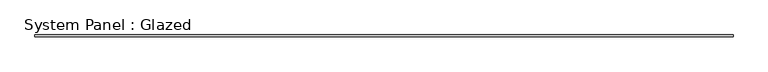
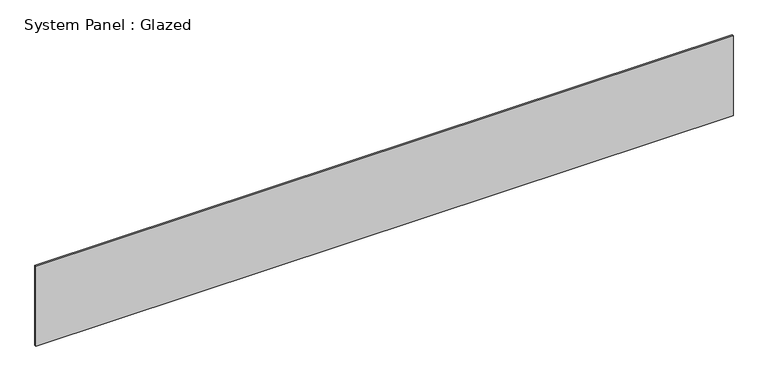
"""IFC4 building model written with IfcOpenShell, lengths in millimetres: plate geometry, System Panel : Glazed."""

from ifc_helpers import new_model, si_unit, origin, origin_with_axes, place, context, project, spatial, polyline, outline, extrude, source, transform, mapped, element, save


def system_panel_glazed_4fccefc8(model_context):
    return source(origin(), model_context, "Body", "SweptSolid", [
        extrude(outline(polyline([(5041.9, 19.05), (-5041.9, 19.05), (-5041.9, 44.45), (5041.9, 44.45), (5041.9, 19.05)])), origin_with_axes(), (0.0, 0.0, 1.0), 1219.2),
    ])


if __name__ == "__main__":
    model = new_model("IFC4")
    model_context = context("Model", 3, world=origin())
    ifc_project = project(units=[si_unit("LENGTHUNIT", "METRE", prefix="MILLI")], contexts=[model_context])
    site = spatial("IfcSite", under=ifc_project)
    building = spatial("IfcBuilding", under=site)
    placement = place(None, origin())
    system_panel_glazed_shape = system_panel_glazed_4fccefc8(model_context)
    element("IfcPlate", 1, ObjectType="System Panel : Glazed", at=placement, inside=building, context=model_context, shape_type="MappedRepresentation", body=[
        mapped(system_panel_glazed_shape, transform((0.0, 0.0, 0.0), x_axis=(1.0, 0.0, 0.0), y_axis=(0.0, 1.0, 0.0), z_axis=(0.0, 0.0, 1.0))),
    ])
    save(model, "model.ifc")

# Revit data of these elements
# Type "System Panel : Glazed"
#   Construction Type Id = "GSP4R"
#   Analytic Construction = "1/8 in Pilkington single glazing"
#   Visual Light Transmittance = 0.9
#   Solar Heat Gain Coefficient = 0.86
#   Heat Transfer Coefficient (U) = 1.18115 BTU/(h·ft²·°F)
# Element 1 (IfcPlate, "System Panel : Glazed")
#   Materials on its faces: "Glass"
# Materials
#   "Glass": class "Glass", colour RGB 0 128 192, transparency 0.75, Description = "Soda Lime Glass", Cost = 0
